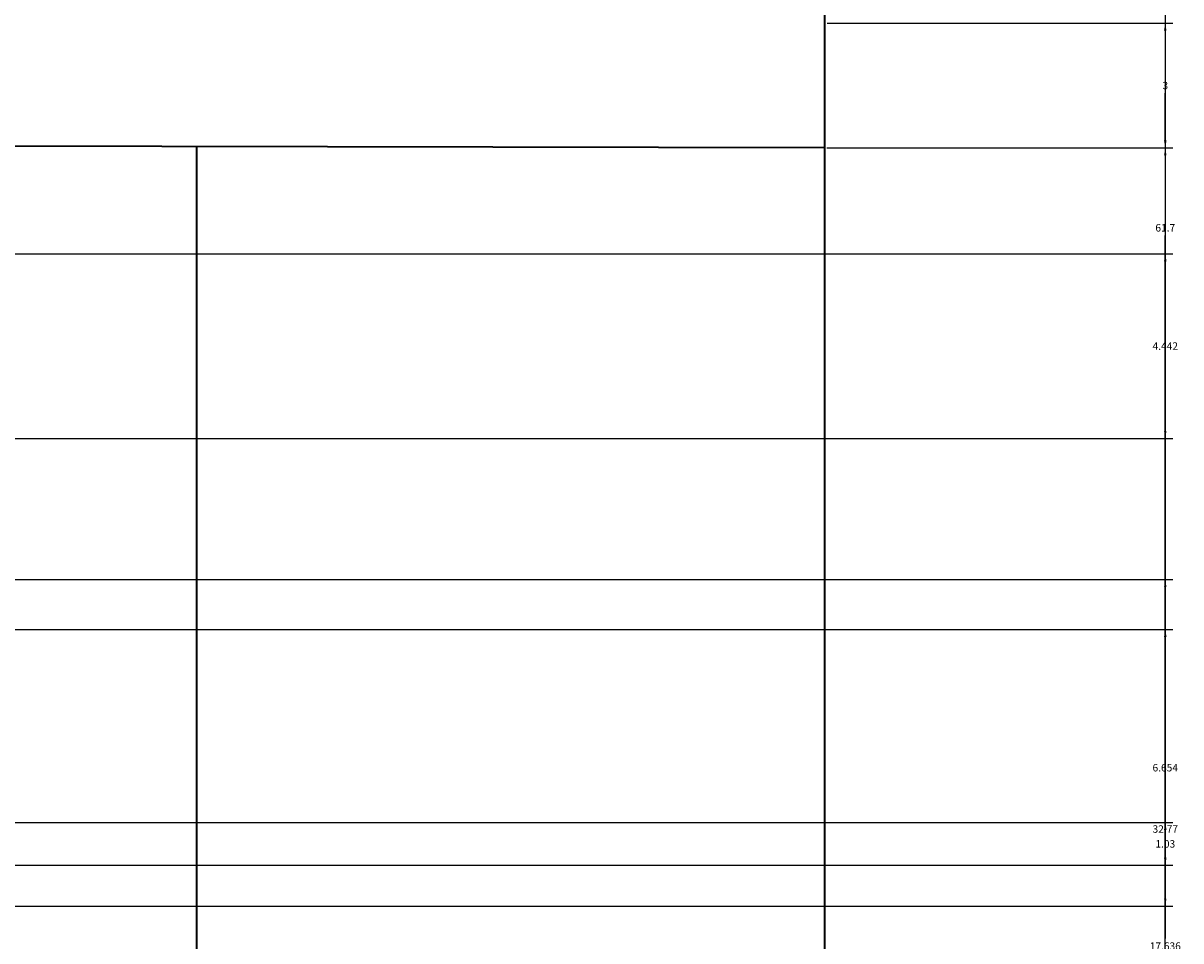
# Model space of a CAD drawing. Units: inches. Extents: x 27 to 200, y -50 to 102.
# Tile 15 of 26: x 172 to 200, y -3 to 19. Entities that reach past the tile are written whole.
import ezdxf

# ---------------------------------------------------------------- set-up
doc = ezdxf.new("R2010")
doc.units = ezdxf.units.IN
doc.header["$MEASUREMENT"] = 0
doc.layers.add('A-ANNO-DIMS', color=2, linetype='Continuous', lineweight=18)
doc.layers.add('A-ELEV', color=7, linetype='Continuous', lineweight=35)
doc.styles.get("Standard").update_dxf_attribs({"font": 'arial.ttf'})
doc.dimstyles.get("Standard").update_dxf_attribs({"dimtxt": 0.18, "dimasz": 0.18, "dimexe": 0.18, "dimexo": 0.0625, "dimgap": 0.09, "dimtad": 0, "dimtih": 1, "dimtoh": 1, "dimdec": 4, "dimzin": 0, "dimdsep": 46, "dimtxsty": 'Standard', "dimcen": 0.09, "dimadec": 0, "dimazin": 0, "dimtfac": 1, "dimtdec": 4, "dimtofl": 0, "dimtmove": 0, "dimatfit": 3, "dimfxl": 1, "dimtolj": 1, "dimtzin": 0, "dimarcsym": 0})

# ---------------------------------------------------------------- blocks, each defined once
blk = doc.blocks.new('*D25')
at = {"layer": 'A-ANNO-DIMS', "color": 0, "lineweight": -2, "transparency": 16777216}
for p, q in [((191.473, 16.002), (199.797, 16.002)), ((199.617, 15.822), (199.617, -0.202)), ((199.617, -16.589), (199.617, -0.566)), ((191.479, -16.769), (199.797, -16.769))]:
    blk.add_line(p, q, dxfattribs=at)
at = {"layer": 'A-ANNO-DIMS', "color": 0, "transparency": 16777216}
for points in [[(199.587, 15.822), (199.647, 15.822), (199.617, 16.002)], [(199.587, -16.589), (199.647, -16.589), (199.617, -16.769)]]:
    blk.add_solid(points, dxfattribs=at)
at = {"layer": 'Defpoints', "color": 0, "transparency": 16777216}
for p in [(191.41, 16.002), (199.617, 16.002), (191.417, -16.769)]:
    blk.add_point(p, dxfattribs=at)
at = {"layer": 'A-ANNO-DIMS', "color": 0, "transparency": 16777216, "insert": (199.617, -0.384), "char_height": 0.18, "attachment_point": 5}
blk.add_mtext('\\A1;32.77', dxfattribs=at)
blk = doc.blocks.new('*D26')
at = {"layer": 'A-ANNO-DIMS', "color": 0, "lineweight": -2, "transparency": 16777216}
for p, q in [((191.479, 19.002), (199.797, 19.002)), ((199.617, 18.822), (199.617, 17.684)), ((199.617, 16.182), (199.617, 17.32)), ((191.473, 16.002), (199.797, 16.002))]:
    blk.add_line(p, q, dxfattribs=at)
at = {"layer": 'A-ANNO-DIMS', "color": 0, "transparency": 16777216}
for points in [[(199.587, 18.822), (199.647, 18.822), (199.617, 19.002)], [(199.587, 16.182), (199.647, 16.182), (199.617, 16.002)]]:
    blk.add_solid(points, dxfattribs=at)
at = {"layer": 'Defpoints', "color": 0, "transparency": 16777216}
for p in [(191.417, 19.002), (199.617, 19.002), (191.41, 16.002)]:
    blk.add_point(p, dxfattribs=at)
at = {"layer": 'A-ANNO-DIMS', "color": 0, "transparency": 16777216, "insert": (199.617, 17.502), "char_height": 0.18, "attachment_point": 5}
blk.add_mtext('\\A1;3', dxfattribs=at)
blk = doc.blocks.new('*D48')
at = {"layer": 'A-ANNO-DIMS', "color": 0, "lineweight": -2, "transparency": 16777216}
for p, q in [((84.479, 44.926), (199.797, 44.926)), ((199.617, 44.746), (199.617, 14.26)), ((199.617, -16.589), (199.617, 13.897)), ((84.479, -16.769), (199.797, -16.769))]:
    blk.add_line(p, q, dxfattribs=at)
at = {"layer": 'A-ANNO-DIMS', "color": 0, "transparency": 16777216}
for points in [[(199.587, 44.746), (199.647, 44.746), (199.617, 44.926)], [(199.587, -16.589), (199.647, -16.589), (199.617, -16.769)]]:
    blk.add_solid(points, dxfattribs=at)
at = {"layer": 'Defpoints', "color": 0, "transparency": 16777216}
for p in [(84.417, 44.926), (199.617, 44.926), (84.417, -16.769)]:
    blk.add_point(p, dxfattribs=at)
at = {"layer": 'A-ANNO-DIMS', "color": 0, "transparency": 16777216, "insert": (199.617, 14.079), "char_height": 0.18, "attachment_point": 5}
blk.add_mtext('\\A1;61.7', dxfattribs=at)
blk = doc.blocks.new('*D58')
at = {"layer": 'A-ANNO-DIMS', "color": 0, "lineweight": -2, "transparency": 16777216}
for p, q in [((140.203, 4.418), (199.797, 4.418)), ((199.617, 4.238), (199.617, 1.273)), ((199.617, -2.056), (199.617, 0.909)), ((140.203, -2.236), (199.797, -2.236))]:
    blk.add_line(p, q, dxfattribs=at)
at = {"layer": 'A-ANNO-DIMS', "color": 0, "transparency": 16777216}
for points in [[(199.587, 4.238), (199.647, 4.238), (199.617, 4.418)], [(199.587, -2.056), (199.647, -2.056), (199.617, -2.236)]]:
    blk.add_solid(points, dxfattribs=at)
at = {"layer": 'Defpoints', "color": 0, "transparency": 16777216}
for p in [(140.141, 4.418), (199.617, 4.418), (140.141, -2.236)]:
    blk.add_point(p, dxfattribs=at)
at = {"layer": 'A-ANNO-DIMS', "color": 0, "transparency": 16777216, "insert": (199.617, 1.091), "char_height": 0.18, "attachment_point": 5}
blk.add_mtext('\\A1;6.654', dxfattribs=at)
blk = doc.blocks.new('*D60')
at = {"layer": 'A-ANNO-DIMS', "color": 0, "lineweight": -2, "transparency": 16777216}
for p, q in [((135.04, -0.225), (199.797, -0.225)), ((199.617, -0.405), (199.617, -0.559)), ((199.617, -1.076), (199.617, -0.923)), ((135.04, -1.256), (199.797, -1.256))]:
    blk.add_line(p, q, dxfattribs=at)
at = {"layer": 'A-ANNO-DIMS', "color": 0, "transparency": 16777216}
for points in [[(199.587, -0.405), (199.647, -0.405), (199.617, -0.225)], [(199.587, -1.076), (199.647, -1.076), (199.617, -1.256)]]:
    blk.add_solid(points, dxfattribs=at)
at = {"layer": 'Defpoints', "color": 0, "transparency": 16777216}
for p in [(134.978, -0.225), (199.617, -0.225), (134.978, -1.256)]:
    blk.add_point(p, dxfattribs=at)
at = {"layer": 'A-ANNO-DIMS', "color": 0, "transparency": 16777216, "insert": (199.617, -0.741), "char_height": 0.18, "attachment_point": 5}
blk.add_mtext('\\A1;1.03', dxfattribs=at)
blk = doc.blocks.new('*D65')
at = {"layer": 'A-ANNO-DIMS', "color": 0, "lineweight": -2, "transparency": 16777216}
for p, q in [((165.546, 13.455), (199.797, 13.455)), ((199.617, 13.275), (199.617, 11.414)), ((199.617, 9.193), (199.617, 11.054)), ((165.546, 9.013), (199.797, 9.013))]:
    blk.add_line(p, q, dxfattribs=at)
at = {"layer": 'A-ANNO-DIMS', "color": 0, "transparency": 16777216}
for points in [[(199.587, 13.275), (199.647, 13.275), (199.617, 13.455)], [(199.587, 9.193), (199.647, 9.193), (199.617, 9.013)]]:
    blk.add_solid(points, dxfattribs=at)
at = {"layer": 'Defpoints', "color": 0, "transparency": 16777216}
for p in [(165.483, 13.455), (199.617, 13.455), (165.483, 9.013)]:
    blk.add_point(p, dxfattribs=at)
at = {"layer": 'A-ANNO-DIMS', "color": 0, "transparency": 16777216, "insert": (199.617, 11.234), "char_height": 0.18, "attachment_point": 5}
blk.add_mtext('\\A1;4.442', dxfattribs=at)
blk = doc.blocks.new('*D67')
at = {"layer": 'A-ANNO-DIMS', "color": 0, "lineweight": -2, "transparency": 16777216}
for p, q in [((165.546, 5.617), (199.797, 5.617)), ((199.617, 5.437), (199.617, -3.019)), ((199.617, -11.839), (199.617, -3.383)), ((165.546, -12.019), (199.797, -12.019))]:
    blk.add_line(p, q, dxfattribs=at)
at = {"layer": 'A-ANNO-DIMS', "color": 0, "transparency": 16777216}
for points in [[(199.587, 5.437), (199.647, 5.437), (199.617, 5.617)], [(199.587, -11.839), (199.647, -11.839), (199.617, -12.019)]]:
    blk.add_solid(points, dxfattribs=at)
at = {"layer": 'Defpoints', "color": 0, "transparency": 16777216}
for p in [(165.484, 5.617), (199.617, 5.617), (165.484, -12.019)]:
    blk.add_point(p, dxfattribs=at)
at = {"layer": 'A-ANNO-DIMS', "color": 0, "transparency": 16777216, "insert": (199.617, -3.201), "char_height": 0.18, "attachment_point": 5}
blk.add_mtext('\\A1;17.636', dxfattribs=at)

msp = doc.modelspace()

# ---------------------------------------------------------------- linework, layer by layer
at = {"layer": 'A-ELEV'}
for p, q in [((191.4169, 93.9264), (191.4169, -16.7693)), ((191.4102, 16.002), (89.3051, 16.2307)), ((176.3118, -16.7693), (176.3118, 16.0358))]:
    msp.add_line(p, q, dxfattribs=at)

# ---------------------------------------------------------------- dimensions: what is measured, and where the dimension line sits
at = {"layer": 'A-ANNO-DIMS'}
for base, p1, p2, override, picture, middle in [((199.6169, 44.9264), (84.4169, -16.7693), (84.4169, 44.9264), {"dimdec": 1, "dimlfac": 1, "dimrnd": 0, "dimzin": 0, "dimdsep": 46, "dimlunit": 2}, '*D48', (199.6169, 14.0786)), ((199.6169, 19.002), (191.4102, 16.002), (191.4169, 19.002), {"dimdec": 0, "dimlfac": 1, "dimrnd": 0, "dimzin": 0, "dimdsep": 46, "dimlunit": 2}, '*D26', (199.6169, 17.502)), ((199.6169, 16.002), (191.4169, -16.7693), (191.4102, 16.002), {"dimdec": 2, "dimlfac": 1, "dimrnd": 0, "dimzin": 0, "dimdsep": 46, "dimlunit": 2}, '*D25', (199.6169, -0.3836)), ((199.6169, 13.4548), (165.4832, 9.0132), (165.4832, 13.4548), {"dimdec": 3, "dimlfac": 1, "dimrnd": 0, "dimzin": 0, "dimdsep": 46, "dimlunit": 2}, '*D65', (199.6169, 11.234)), ((199.6169, 5.6167), (165.4839, -12.0191), (165.4839, 5.6167), {"dimdec": 3, "dimlfac": 1, "dimrnd": 0, "dimzin": 0, "dimdsep": 46, "dimlunit": 2}, '*D67', (199.6169, -3.2012)), ((199.6169, 4.4177), (140.1406, -2.2364), (140.1406, 4.4177), {"dimdec": 3, "dimlfac": 1, "dimrnd": 0, "dimzin": 0, "dimdsep": 46, "dimlunit": 2}, '*D58', (199.6169, 1.0906)), ((199.6169, -0.2247), (134.9776, -1.2564), (134.9776, -0.2247), {"dimdec": 2, "dimlfac": 1, "dimrnd": 0, "dimzin": 0, "dimdsep": 46, "dimlunit": 2}, '*D60', (199.6169, -0.7405))]:
    dim = msp.add_linear_dim(base=base, p1=p1, p2=p2, angle=90, dimstyle='Standard', override=override, dxfattribs=at)
    dim.commit()
    dim.dimension.update_dxf_attribs({"geometry": picture, "text_midpoint": middle})

doc.saveas('drawing.dxf')
